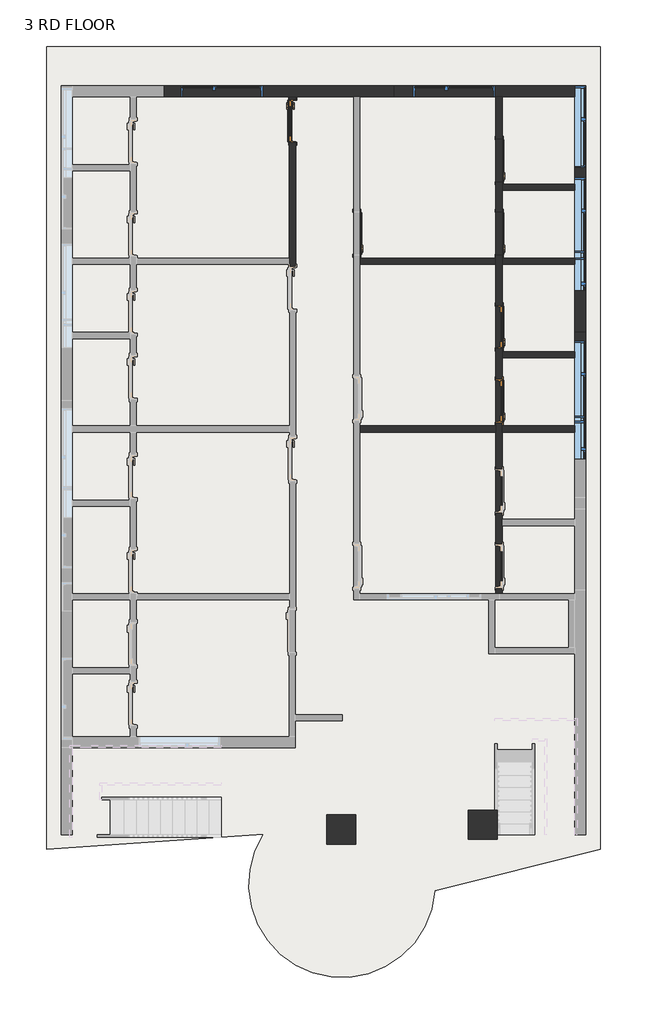
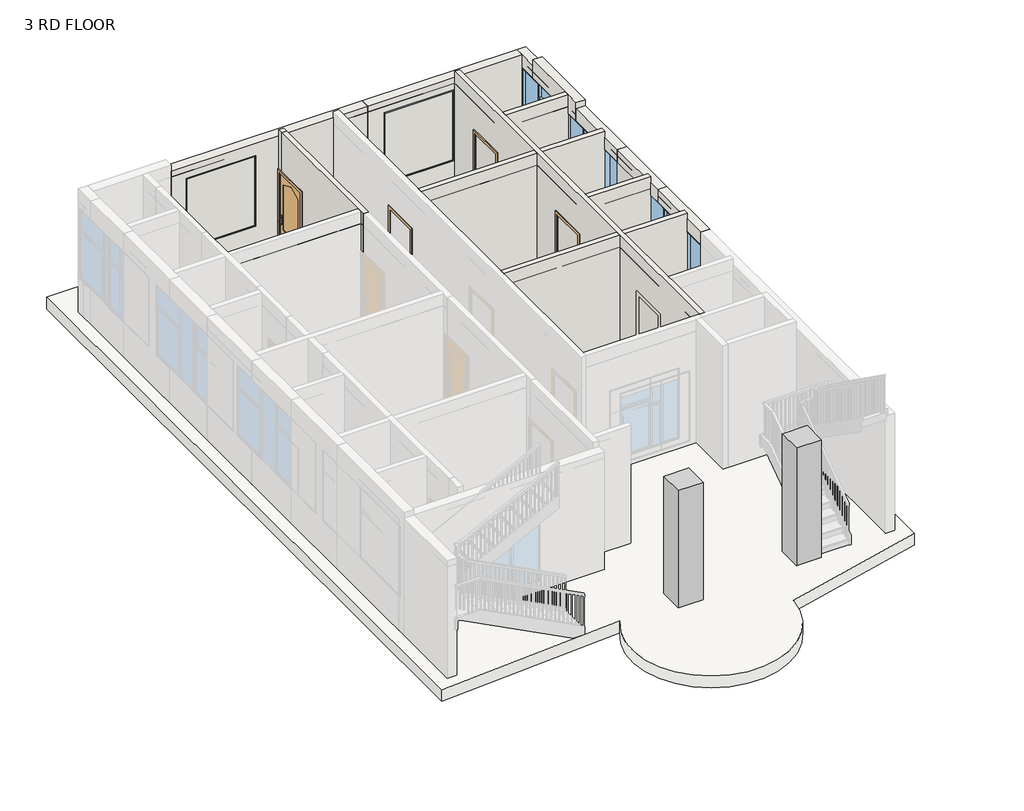
# One storey, part 3 of 5: 33 walls, 7 windows, 6 doors, 2 columns, 1 slab.
"""IFC4 building model written with IfcOpenShell, lengths in millimetres."""

from ifc_helpers import new_model, si_unit, point, frame, frame_2d, origin, place, context, project, spatial, polyline, circle_curve, trimmed, segment, composite_curve, outline, extrude, faceted_brep, transform, mapped, element, save
from components import column_08700e81, door_346b4a94, m_window_casement_double_sidelight_1702_x_1829mm_c8b42c7f

model = new_model("IFC4")

# Units and contexts
model_context = context("Model", 3, world=origin())
ifc_project = project(units=[si_unit("LENGTHUNIT", "METRE", prefix="MILLI")], contexts=[model_context])

# Site, building, storey
site = spatial("IfcSite", under=ifc_project)
building = spatial("IfcBuilding", under=site)
storey = spatial("IfcBuildingStorey", under=building, Name="3 RD FLOOR", Elevation=9601.2)

# Columns
placement = place(None, origin())
element("IfcColumn", 1, ObjectType="Rectangular Column : 24\" x 24\"", at=placement, inside=storey, context=model_context, shape_type="SweptSolid", body=[
    extrude(outline(polyline([(2657.4891134, -7132.8082131), (2657.4891134, -7742.4082131), (2047.8891134, -7742.4082131), (2047.8891134, -7132.8082131), (2657.4891134, -7132.8082131)])), frame((0.0, 0.0, 9601.2), z_axis=(0.0, 0.0, 1.0), x_axis=(1.0, 0.0, 0.0)), (0.0, 0.0, 1.0), 3048.0),
])
column_shape = column_08700e81(model_context)
element("IfcColumn", 2, ObjectType="Rectangular Column : 24\" x 24\"", at=placement, inside=storey, context=model_context, shape_type="MappedRepresentation", body=[
    mapped(column_shape, transform((-606.4108866, -7539.2082131, 0.0), x_axis=(1.0, 0.0, 0.0), y_axis=(0.0, 1.0, 0.0), z_axis=(0.0, 0.0, 1.0))),
])

# Doors
door_shape = door_346b4a94(model_context)
element("IfcDoor", 3, ObjectType="2'10\"X7'", at=placement, inside=storey, context=model_context, shape_type="MappedRepresentation", body=[
    mapped(door_shape, transform((2698.7641134, 6449.4399728, 9601.2), x_axis=(0.0, -1.0, 0.0), y_axis=(1.0, 0.0, 0.0), z_axis=(0.0, 0.0, 1.0))),
])
element("IfcDoor", 4, ObjectType="2'10\"X7'", at=placement, inside=storey, context=model_context, shape_type="MappedRepresentation", body=[
    mapped(door_shape, transform((2698.7641134, 4925.4399728, 9601.2), x_axis=(0.0, -1.0, 0.0), y_axis=(1.0, 0.0, 0.0), z_axis=(0.0, 0.0, 1.0))),
])
element("IfcDoor", 5, ObjectType="2'10\"X7'", at=placement, inside=storey, context=model_context, shape_type="MappedRepresentation", body=[
    mapped(door_shape, transform((2698.7641134, 2969.6399728, 9601.2), x_axis=(0.0, -1.0, 0.0), y_axis=(1.0, 0.0, 0.0), z_axis=(0.0, 0.0, 1.0))),
])
element("IfcDoor", 6, ObjectType="2'10\"X7'", at=placement, inside=storey, context=model_context, shape_type="MappedRepresentation", body=[
    mapped(door_shape, transform((2698.7641134, 1420.2399728, 9601.2), x_axis=(0.0, -1.0, 0.0), y_axis=(1.0, 0.0, 0.0), z_axis=(0.0, 0.0, 1.0))),
])
element("IfcDoor", 7, ObjectType="2'10\"X7'", at=placement, inside=storey, context=model_context, shape_type="MappedRepresentation", body=[
    mapped(door_shape, transform((-273.0358866, 4925.4399728, 9601.2), x_axis=(0.0, -1.0, 0.0), y_axis=(1.0, 0.0, 0.0), z_axis=(0.0, 0.0, 1.0))),
])
element("IfcDoor", 8, ObjectType="2'10\"X7'", at=placement, inside=storey, context=model_context, shape_type="MappedRepresentation", body=[
    mapped(door_shape, transform((-1625.5858866, 7274.3310623, 9601.2), x_axis=(0.0, 1.0, 0.0), y_axis=(-1.0, 0.0, 0.0), z_axis=(0.0, 0.0, 1.0))),
])

# Slab
element("IfcSlab", 9, ObjectType="Generic - 12\"", at=placement, inside=storey, context=model_context, shape_type="SweptSolid", body=[
    extrude(outline(composite_curve([segment(polyline([(4815.1311655, 8833.6177996), (4815.1311655, -7955.7822004), (1352.4742985, -8819.1195216)]), True, "CONTINUOUS"), segment(trimmed(circle_curve(frame_2d((-589.5644815, -8685.9789369)), 1946.5972974), [point((1352.4742985, -8819.1195216))], [point((-2230.3861756, -7638.6274169))], False, "CARTESIAN"), True, "CONTINUOUS"), segment(polyline([(-2230.3861756, -7638.6274169), (-6765.9108866, -7955.7822004), (-6765.9108866, 8833.6177996), (4815.1311655, 8833.6177996)]), True, "CONTINUOUS")], self_intersect=False)), frame((0.0, 0.0, 9296.4), z_axis=(0.0, 0.0, 1.0), x_axis=(1.0, 0.0, 0.0)), (0.0, 0.0, 1.0), 304.8),
])

# Walls
element("IfcWall", 10, ObjectType="Generic - 4.5\"", at=placement, inside=storey, context=model_context, shape_type="Brep", body=[
    faceted_brep([(-1685.9108866, 7655.3310623, 12801.6), (-1685.9108866, 7782.9399728, 12801.6), (-1685.9108866, 7782.9399728, 9601.2), (-1685.9108866, 7731.1310623, 9601.2), (-1685.9108866, 7731.1310623, 11759.8), (-1685.9108866, 7655.3310623, 11759.8), (-1685.9108866, 7655.3310623, 12496.8), (-1558.9108866, 7782.9399728, 12801.6), (-1558.9108866, 7655.3310623, 12801.6), (-1558.9108866, 7655.3310623, 12496.8), (-1558.9108866, 7655.3310623, 11759.8), (-1558.9108866, 7731.1310623, 11759.8), (-1558.9108866, 7731.1310623, 9601.2), (-1558.9108866, 7782.9399728, 9601.2)], [[[0, 1, 2, 3, 4, 5, 6]], [[7, 8, 9, 10, 11, 12, 13]], [[2, 13, 12, 3]], [[1, 0, 8, 7]], [[11, 4, 3, 12]], [[4, 11, 10, 5]], [[8, 0, 6, 5, 10, 9]], [[1, 7, 13, 2]]]),
])
element("IfcWall", 11, ObjectType="Generic - 4.5\"", at=placement, inside=storey, context=model_context, shape_type="Brep", body=[
    faceted_brep([(-1685.9108866, 4182.2008884, 12801.6), (-1685.9108866, 4277.7399728, 12801.6), (-1685.9108866, 4404.7399728, 12801.6), (-1685.9108866, 7655.3310623, 12801.6), (-1685.9108866, 7655.3310623, 12496.8), (-1685.9108866, 7655.3310623, 11759.8), (-1685.9108866, 6817.5310623, 11759.8), (-1685.9108866, 6817.5310623, 9601.2), (-1685.9108866, 4404.7399728, 9601.2), (-1685.9108866, 4277.7399728, 9601.2), (-1685.9108866, 4232.6008884, 9601.2), (-1685.9108866, 4232.6008884, 11759.8), (-1685.9108866, 4182.2008884, 11759.8), (-1558.9108866, 7655.3310623, 12801.6), (-1558.9108866, 4182.2008884, 12801.6), (-1558.9108866, 4182.2008884, 11759.8), (-1558.9108866, 4232.6008884, 11759.8), (-1558.9108866, 4232.6008884, 9601.2), (-1558.9108866, 6817.5310623, 9601.2), (-1558.9108866, 6817.5310623, 11759.8), (-1558.9108866, 7655.3310623, 11759.8), (-1558.9108866, 7655.3310623, 12496.8), (-1685.4871817, 4182.2008884, 12801.6), (-1685.4871817, 4182.2008884, 11759.8)], [[[0, 1, 2, 3, 4, 5, 6, 7, 8, 9, 10, 11, 12]], [[13, 14, 15, 16, 17, 18, 19, 20, 21]], [[17, 10, 9, 8, 7, 18]], [[3, 2, 1, 0, 22, 14, 13]], [[16, 11, 10, 17]], [[11, 16, 15, 23, 12]], [[19, 6, 5, 20]], [[6, 19, 18, 7]], [[14, 22, 0, 12, 23, 15]], [[3, 13, 21, 20, 5, 4]]]),
])
element("IfcWall", 12, ObjectType="Generic - 4.5\"", at=placement, inside=storey, context=model_context, shape_type="Brep", body=[
    faceted_brep([(2632.0891134, -2605.6600272, 12801.6), (2632.0891134, 772.5399728, 12801.6), (2632.0891134, 899.5399728, 12801.6), (2632.0891134, 4277.7399728, 12801.6), (2632.0891134, 4404.7399728, 12801.6), (2632.0891134, 7782.9399728, 12801.6), (2632.0891134, 7782.9399728, 9601.2), (2632.0891134, 6906.2399728, 9601.2), (2632.0891134, 6906.2399728, 11759.8), (2632.0891134, 5992.6399728, 11759.8), (2632.0891134, 5992.6399728, 9601.2), (2632.0891134, 5382.2399728, 9601.2), (2632.0891134, 5382.2399728, 11759.8), (2632.0891134, 4468.6399728, 11759.8), (2632.0891134, 4468.6399728, 9601.2), (2632.0891134, 4404.7399728, 9601.2), (2632.0891134, 4277.7399728, 9601.2), (2632.0891134, 3426.4399728, 9601.2), (2632.0891134, 3426.4399728, 11759.8), (2632.0891134, 2512.8399728, 11759.8), (2632.0891134, 2512.8399728, 9601.2), (2632.0891134, 1877.0399728, 9601.2), (2632.0891134, 1877.0399728, 11759.8), (2632.0891134, 963.4399728, 11759.8), (2632.0891134, 963.4399728, 9601.2), (2632.0891134, 899.5399728, 9601.2), (2632.0891134, 772.5399728, 9601.2), (2632.0891134, -2.5600272, 9601.2), (2632.0891134, -2.5600272, 11759.8), (2632.0891134, -916.1600272, 11759.8), (2632.0891134, -916.1600272, 9601.2), (2632.0891134, -1577.3600272, 9601.2), (2632.0891134, -1577.3600272, 11759.8), (2632.0891134, -2490.9600272, 11759.8), (2632.0891134, -2490.9600272, 9601.2), (2632.0891134, -2605.6600272, 9601.2), (2632.0891134, -2605.6600272, 12496.8), (2759.0891134, 7782.9399728, 12801.6), (2759.0891134, 5954.1399728, 12801.6), (2759.0891134, 5827.1399728, 12801.6), (2759.0891134, 4404.7399728, 12801.6), (2759.0891134, 4277.7399728, 12801.6), (2759.0891134, 2448.9399728, 12801.6), (2759.0891134, 2321.9399728, 12801.6), (2759.0891134, 899.5399728, 12801.6), (2759.0891134, 772.5399728, 12801.6), (2759.0891134, -1056.2600272, 12801.6), (2759.0891134, -1183.2600272, 12801.6), (2759.0891134, -2605.6600272, 12801.6), (2759.0891134, -2605.6600272, 9601.2), (2759.0891134, -2490.9600272, 9601.2), (2759.0891134, -2490.9600272, 11759.8), (2759.0891134, -1577.3600272, 11759.8), (2759.0891134, -1577.3600272, 9601.2), (2759.0891134, -1183.2600272, 9601.2), (2759.0891134, -1056.2600272, 9601.2), (2759.0891134, -916.1600272, 9601.2), (2759.0891134, -916.1600272, 11759.8), (2759.0891134, -2.5600272, 11759.8), (2759.0891134, -2.5600272, 9601.2), (2759.0891134, 772.5399728, 9601.2), (2759.0891134, 899.5399728, 9601.2), (2759.0891134, 963.4399728, 9601.2), (2759.0891134, 963.4399728, 11759.8), (2759.0891134, 1877.0399728, 11759.8), (2759.0891134, 1877.0399728, 9601.2), (2759.0891134, 2321.9399728, 9601.2), (2759.0891134, 2448.9399728, 9601.2), (2759.0891134, 2512.8399728, 9601.2), (2759.0891134, 2512.8399728, 11759.8), (2759.0891134, 3426.4399728, 11759.8), (2759.0891134, 3426.4399728, 9601.2), (2759.0891134, 4277.7399728, 9601.2), (2759.0891134, 4404.7399728, 9601.2), (2759.0891134, 4468.6399728, 9601.2), (2759.0891134, 4468.6399728, 11759.8), (2759.0891134, 5382.2399728, 11759.8), (2759.0891134, 5382.2399728, 9601.2), (2759.0891134, 5827.1399728, 9601.2), (2759.0891134, 5954.1399728, 9601.2), (2759.0891134, 5992.6399728, 9601.2), (2759.0891134, 5992.6399728, 11759.8), (2759.0891134, 6906.2399728, 11759.8), (2759.0891134, 6906.2399728, 9601.2), (2759.0891134, 7782.9399728, 9601.2), (2695.5891134, -2605.6600272, 9601.2)], [[[0, 1, 2, 3, 4, 5, 6, 7, 8, 9, 10, 11, 12, 13, 14, 15, 16, 17, 18, 19, 20, 21, 22, 23, 24, 25, 26, 27, 28, 29, 30, 31, 32, 33, 34, 35, 36]], [[37, 38, 39, 40, 41, 42, 43, 44, 45, 46, 47, 48, 49, 50, 51, 52, 53, 54, 55, 56, 57, 58, 59, 60, 61, 62, 63, 64, 65, 66, 67, 68, 69, 70, 71, 72, 73, 74, 75, 76, 77, 78, 79, 80, 81, 82, 83, 84]], [[6, 84, 83, 7]], [[10, 80, 79, 78, 77, 11]], [[14, 74, 73, 72, 71, 17, 16, 15]], [[20, 68, 67, 66, 65, 21]], [[24, 62, 61, 60, 59, 27, 26, 25]], [[30, 56, 55, 54, 53, 31]], [[49, 85, 35, 34, 50]], [[5, 4, 3, 2, 1, 0, 48, 47, 46, 45, 44, 43, 42, 41, 40, 39, 38, 37]], [[6, 5, 37, 84]], [[9, 81, 80, 10]], [[81, 9, 8, 82]], [[82, 8, 7, 83]], [[14, 13, 75, 74]], [[13, 12, 76, 75]], [[12, 11, 77, 76]], [[19, 69, 68, 20]], [[69, 19, 18, 70]], [[70, 18, 17, 71]], [[23, 63, 62, 24]], [[63, 23, 22, 64]], [[64, 22, 21, 65]], [[29, 57, 56, 30]], [[57, 29, 28, 58]], [[58, 28, 27, 59]], [[33, 51, 50, 34]], [[51, 33, 32, 52]], [[52, 32, 31, 53]], [[35, 85, 49, 48, 0, 36]]]),
])
element("IfcWall", 13, ObjectType="Generic - 4.5\"", at=placement, inside=storey, context=model_context, shape_type="SweptSolid", body=[
    extrude(outline(polyline([(2632.0891134, 4277.7399728), (-212.7108866, 4277.7399728), (-212.7108866, 4404.7399728), (2632.0891134, 4404.7399728), (2632.0891134, 4277.7399728)])), frame((0.0, 0.0, 9601.2), z_axis=(0.0, 0.0, 1.0), x_axis=(1.0, 0.0, 0.0)), (0.0, 0.0, 1.0), 3200.4),
])
element("IfcWall", 14, ObjectType="Generic - 4.5\"", at=placement, inside=storey, context=model_context, shape_type="SweptSolid", body=[
    extrude(outline(polyline([(2632.0891134, 772.5399728), (-212.7108866, 772.5399728), (-212.7108866, 899.5399728), (2632.0891134, 899.5399728), (2632.0891134, 772.5399728)])), frame((0.0, 0.0, 9601.2), z_axis=(0.0, 0.0, 1.0), x_axis=(1.0, 0.0, 0.0)), (0.0, 0.0, 1.0), 3200.4),
])
element("IfcWall", 15, ObjectType="Generic - 4.5\"", at=placement, inside=storey, context=model_context, shape_type="SweptSolid", body=[
    extrude(outline(polyline([(4281.587404, 5827.1399728), (2759.0891134, 5827.1399728), (2759.0891134, 5954.1399728), (4281.587404, 5954.1399728), (4281.587404, 5827.1399728)])), frame((0.0, 0.0, 9601.2), z_axis=(0.0, 0.0, 1.0), x_axis=(1.0, 0.0, 0.0)), (0.0, 0.0, 1.0), 3200.4),
])
element("IfcWall", 16, ObjectType="Generic - 4.5\"", at=placement, inside=storey, context=model_context, shape_type="SweptSolid", body=[
    extrude(outline(polyline([(4283.9989713, 4277.7399728), (2759.0891134, 4277.7399728), (2759.0891134, 4404.7399728), (4283.9989713, 4404.7399728), (4283.9989713, 4277.7399728)])), frame((0.0, 0.0, 9601.2), z_axis=(0.0, 0.0, 1.0), x_axis=(1.0, 0.0, 0.0)), (0.0, 0.0, 1.0), 3200.4),
])
element("IfcWall", 17, ObjectType="Generic - 4.5\"", at=placement, inside=storey, context=model_context, shape_type="SweptSolid", body=[
    extrude(outline(polyline([(4281.0767915, 2321.9399728), (2759.0891134, 2321.9399728), (2759.0891134, 2448.9399728), (4281.0767915, 2448.9399728), (4281.0767915, 2321.9399728)])), frame((0.0, 0.0, 9601.2), z_axis=(0.0, 0.0, 1.0), x_axis=(1.0, 0.0, 0.0)), (0.0, 0.0, 1.0), 3200.4),
])
element("IfcWall", 18, ObjectType="Generic - 4.5\"", at=placement, inside=storey, context=model_context, shape_type="SweptSolid", body=[
    extrude(outline(polyline([(4283.0918814, 772.5399728), (2759.0891134, 772.5399728), (2759.0891134, 899.5399728), (4283.0918814, 899.5399728), (4283.0918814, 772.5399728)])), frame((0.0, 0.0, 9601.2), z_axis=(0.0, 0.0, 1.0), x_axis=(1.0, 0.0, 0.0)), (0.0, 0.0, 1.0), 3200.4),
])
element("IfcWall", 19, ObjectType="Generic - 4.5\"", at=placement, inside=storey, context=model_context, shape_type="SweptSolid", body=[
    extrude(outline(polyline([(-1685.9108866, 4277.7399728), (-4886.3108866, 4277.7399728), (-4886.3108866, 4404.7399728), (-1685.9108866, 4404.7399728), (-1685.9108866, 4277.7399728)])), frame((0.0, 0.0, 9601.2), z_axis=(0.0, 0.0, 1.0), x_axis=(1.0, 0.0, 0.0)), (0.0, 0.0, 1.0), 2895.6),
])
element("IfcWall", 20, ObjectType="Generic - 4.5\"", at=placement, inside=storey, context=model_context, shape_type="SweptSolid", body=[
    extrude(outline(polyline([(7782.9399728, 12496.8), (7782.9399728, 9601.2), (7731.1310623, 9601.2), (7731.1310623, 11759.8), (7655.3310623, 11759.8), (7655.3310623, 12496.8), (7782.9399728, 12496.8)])), frame((-1685.9108866, 0.0, 0.0), z_axis=(1.0, 0.0, 0.0), x_axis=(0.0, 1.0, 0.0)), (0.0, 0.0, 1.0), 127.0),
])
element("IfcWall", 21, ObjectType="Generic - 4.5\"", at=placement, inside=storey, context=model_context, shape_type="Brep", body=[
    faceted_brep([(-1685.9108866, 4182.2008884, 12496.8), (-1685.9108866, 4277.7399728, 12496.8), (-1685.9108866, 4404.7399728, 12496.8), (-1685.9108866, 7655.3310623, 12496.8), (-1685.9108866, 7655.3310623, 11759.8), (-1685.9108866, 6817.5310623, 11759.8), (-1685.9108866, 6817.5310623, 9601.2), (-1685.9108866, 4404.7399728, 9601.2), (-1685.9108866, 4277.7399728, 9601.2), (-1685.9108866, 4232.6008884, 9601.2), (-1685.9108866, 4232.6008884, 11759.8), (-1685.9108866, 4182.2008884, 11759.8), (-1558.9108866, 7655.3310623, 12496.8), (-1558.9108866, 4182.2008884, 12496.8), (-1558.9108866, 4182.2008884, 11759.8), (-1558.9108866, 4232.6008884, 11759.8), (-1558.9108866, 4232.6008884, 9601.2), (-1558.9108866, 6817.5310623, 9601.2), (-1558.9108866, 6817.5310623, 11759.8), (-1558.9108866, 7655.3310623, 11759.8), (-1685.4871817, 4182.2008884, 12496.8), (-1685.4871817, 4182.2008884, 11759.8)], [[[0, 1, 2, 3, 4, 5, 6, 7, 8, 9, 10, 11]], [[12, 13, 14, 15, 16, 17, 18, 19]], [[16, 9, 8, 7, 6, 17]], [[13, 20, 0, 11, 21, 14]], [[3, 12, 19, 4]], [[3, 2, 1, 0, 20, 13, 12]], [[18, 5, 4, 19]], [[5, 18, 17, 6]], [[15, 10, 9, 16]], [[10, 15, 14, 21, 11]]]),
])
element("IfcWall", 22, ObjectType="Generic - 4.5\"", at=placement, inside=storey, context=model_context, shape_type="Brep", body=[
    faceted_brep([(2632.0891134, 7782.9399728, 9601.2), (2632.0891134, 4404.7399728, 9601.2), (2632.0891134, 4277.7399728, 9601.2), (2632.0891134, 899.5399728, 9601.2), (2632.0891134, 772.5399728, 9601.2), (2632.0891134, -2605.6600272, 9601.2), (2632.0891134, -2605.6600272, 12496.8), (2632.0891134, 772.5399728, 12496.8), (2632.0891134, 899.5399728, 12496.8), (2632.0891134, 4277.7399728, 12496.8), (2632.0891134, 4404.7399728, 12496.8), (2632.0891134, 7782.9399728, 12496.8), (2759.0891134, 7782.9399728, 9601.2), (2759.0891134, 7782.9399728, 12496.8), (2759.0891134, 5954.1399728, 12496.8), (2759.0891134, 5827.1399728, 12496.8), (2759.0891134, 4404.7399728, 12496.8), (2759.0891134, 4277.7399728, 12496.8), (2759.0891134, 2448.9399728, 12496.8), (2759.0891134, 2321.9399728, 12496.8), (2759.0891134, 899.5399728, 12496.8), (2759.0891134, 772.5399728, 12496.8), (2759.0891134, -1056.2600272, 12496.8), (2759.0891134, -1183.2600272, 12496.8), (2759.0891134, -2605.6600272, 12496.8), (2759.0891134, -2605.6600272, 9601.2), (2759.0891134, -1183.2600272, 9601.2), (2759.0891134, -1056.2600272, 9601.2), (2759.0891134, 772.5399728, 9601.2), (2759.0891134, 899.5399728, 9601.2), (2759.0891134, 2321.9399728, 9601.2), (2759.0891134, 2448.9399728, 9601.2), (2759.0891134, 4277.7399728, 9601.2), (2759.0891134, 4404.7399728, 9601.2), (2759.0891134, 5827.1399728, 9601.2), (2759.0891134, 5954.1399728, 9601.2), (2695.5891134, -2605.6600272, 9601.2), (2695.5891134, -2605.6600272, 12496.8)], [[[0, 1, 2, 3, 4, 5, 6, 7, 8, 9, 10, 11]], [[12, 13, 14, 15, 16, 17, 18, 19, 20, 21, 22, 23, 24, 25, 26, 27, 28, 29, 30, 31, 32, 33, 34, 35]], [[5, 4, 3, 2, 1, 0, 12, 35, 34, 33, 32, 31, 30, 29, 28, 27, 26, 25, 36]], [[0, 11, 13, 12]], [[6, 5, 36, 25, 24, 37]], [[11, 10, 9, 8, 7, 6, 37, 24, 23, 22, 21, 20, 19, 18, 17, 16, 15, 14, 13]]]),
])
element("IfcWall", 23, ObjectType="Generic - 4.5\"", at=placement, inside=storey, context=model_context, shape_type="SweptSolid", body=[
    extrude(outline(polyline([(2632.0891134, 4277.7399728), (-212.7108866, 4277.7399728), (-212.7108866, 4404.7399728), (2632.0891134, 4404.7399728), (2632.0891134, 4277.7399728)])), frame((0.0, 0.0, 9601.2), z_axis=(0.0, 0.0, 1.0), x_axis=(1.0, 0.0, 0.0)), (0.0, 0.0, 1.0), 2895.6),
])
element("IfcWall", 24, ObjectType="Generic - 4.5\"", at=placement, inside=storey, context=model_context, shape_type="SweptSolid", body=[
    extrude(outline(polyline([(2632.0891134, 772.5399728), (-212.7108866, 772.5399728), (-212.7108866, 899.5399728), (2632.0891134, 899.5399728), (2632.0891134, 772.5399728)])), frame((0.0, 0.0, 9601.2), z_axis=(0.0, 0.0, 1.0), x_axis=(1.0, 0.0, 0.0)), (0.0, 0.0, 1.0), 2895.6),
])
element("IfcWall", 25, ObjectType="Generic - 4.5\"", at=placement, inside=storey, context=model_context, shape_type="SweptSolid", body=[
    extrude(outline(polyline([(4281.587404, 5827.1399728), (2759.0891134, 5827.1399728), (2759.0891134, 5954.1399728), (4281.587404, 5954.1399728), (4281.587404, 5827.1399728)])), frame((0.0, 0.0, 9601.2), z_axis=(0.0, 0.0, 1.0), x_axis=(1.0, 0.0, 0.0)), (0.0, 0.0, 1.0), 2895.6),
])
element("IfcWall", 26, ObjectType="Generic - 4.5\"", at=placement, inside=storey, context=model_context, shape_type="SweptSolid", body=[
    extrude(outline(polyline([(4283.9989713, 4277.7399728), (2759.0891134, 4277.7399728), (2759.0891134, 4404.7399728), (4283.9989713, 4404.7399728), (4283.9989713, 4277.7399728)])), frame((0.0, 0.0, 9601.2), z_axis=(0.0, 0.0, 1.0), x_axis=(1.0, 0.0, 0.0)), (0.0, 0.0, 1.0), 2895.6),
])
element("IfcWall", 27, ObjectType="Generic - 4.5\"", at=placement, inside=storey, context=model_context, shape_type="SweptSolid", body=[
    extrude(outline(polyline([(4281.0767915, 2321.9399728), (2759.0891134, 2321.9399728), (2759.0891134, 2448.9399728), (4281.0767915, 2448.9399728), (4281.0767915, 2321.9399728)])), frame((0.0, 0.0, 9601.2), z_axis=(0.0, 0.0, 1.0), x_axis=(1.0, 0.0, 0.0)), (0.0, 0.0, 1.0), 2895.6),
])
element("IfcWall", 28, ObjectType="Generic - 4.5\"", at=placement, inside=storey, context=model_context, shape_type="SweptSolid", body=[
    extrude(outline(polyline([(4283.0918814, 772.5399728), (2759.0891134, 772.5399728), (2759.0891134, 899.5399728), (4283.0918814, 899.5399728), (4283.0918814, 772.5399728)])), frame((0.0, 0.0, 9601.2), z_axis=(0.0, 0.0, 1.0), x_axis=(1.0, 0.0, 0.0)), (0.0, 0.0, 1.0), 2895.6),
])
element("IfcWall", 29, ObjectType="Generic - 9\"", at=placement, inside=storey, context=model_context, shape_type="Brep", body=[
    faceted_brep([(-4318.2603585, 7782.9399728, 12649.2), (-4318.2603585, 7782.9399728, 12496.8), (-4318.2603585, 7782.9399728, 9601.2), (-1685.9108866, 7782.9399728, 9601.2), (-1558.9108866, 7782.9399728, 9601.2), (-339.7108866, 7782.9399728, 9601.2), (-212.7108866, 7782.9399728, 9601.2), (496.3553976, 7782.9399728, 9601.2), (496.3553976, 7782.9399728, 12496.8), (496.3553976, 7782.9399728, 12649.2), (-2248.1603585, 7782.9399728, 12330.0), (-2248.1603585, 7782.9399728, 10501.2), (-3949.9603585, 7782.9399728, 10501.2), (-3949.9603585, 7782.9399728, 12330.0), (-4318.2603585, 8011.5399728, 9601.2), (-4318.2603585, 8011.5399728, 12496.8), (-4318.2603585, 8011.5399728, 12649.2), (496.3553976, 8011.5399728, 12649.2), (496.3553976, 8011.5399728, 12496.8), (496.3553976, 8011.5399728, 9601.2), (-2248.1603585, 8011.5399728, 12330.0), (-3949.9603585, 8011.5399728, 12330.0), (-3949.9603585, 8011.5399728, 10501.2), (-2248.1603585, 8011.5399728, 10501.2)], [[[0, 1, 2, 3, 4, 5, 6, 7, 8, 9], [10, 11, 12, 13]], [[14, 15, 16, 17, 18, 19], [20, 21, 22, 23]], [[7, 6, 5, 4, 3, 2, 14, 19]], [[0, 9, 17, 16]], [[11, 10, 20, 23]], [[12, 11, 23, 22]], [[13, 12, 22, 21]], [[10, 13, 21, 20]], [[7, 19, 18, 17, 9, 8]], [[0, 16, 15, 14, 2, 1]]]),
])
element("IfcWall", 30, ObjectType="Generic - 9\"", at=placement, inside=storey, context=model_context, shape_type="Brep", body=[
    faceted_brep([(496.3553976, 7782.9399728, 9601.2), (2632.0891134, 7782.9399728, 9601.2), (2759.0891134, 7782.9399728, 9601.2), (4283.0891134, 7782.9399728, 9601.2), (4283.0891134, 7782.9399728, 10501.2), (4281.587404, 7782.9399728, 10501.2), (4281.587404, 7782.9399728, 12330.0), (4283.0891134, 7782.9399728, 12330.0), (4283.0891134, 7782.9399728, 12649.2), (496.3553976, 7782.9399728, 12649.2), (496.3553976, 7782.9399728, 12496.8), (2606.6891134, 7782.9399728, 12330.0), (2606.6891134, 7782.9399728, 10501.2), (904.8891134, 7782.9399728, 10501.2), (904.8891134, 7782.9399728, 12330.0), (4283.0891134, 8011.5399728, 9601.2), (496.3553976, 8011.5399728, 9601.2), (496.3553976, 8011.5399728, 12496.8), (496.3553976, 8011.5399728, 12649.2), (4283.0891134, 8011.5399728, 12649.2), (4283.0891134, 8011.5399728, 12496.8), (2606.6891134, 8011.5399728, 10501.2), (2606.6891134, 8011.5399728, 12330.0), (904.8891134, 8011.5399728, 12330.0), (904.8891134, 8011.5399728, 10501.2), (4283.0891134, 7998.8399728, 12330.0), (4283.0891134, 7998.8399728, 10501.2), (4281.587404, 7998.8399728, 10501.2), (4281.587404, 7998.8399728, 12330.0)], [[[0, 1, 2, 3, 4, 5, 6, 7, 8, 9, 10], [11, 12, 13, 14]], [[15, 16, 17, 18, 19, 20], [21, 22, 23, 24]], [[3, 2, 1, 0, 16, 15]], [[9, 8, 19, 18]], [[12, 11, 22, 21]], [[13, 12, 21, 24]], [[14, 13, 24, 23]], [[11, 14, 23, 22]], [[9, 18, 17, 16, 0, 10]], [[3, 15, 20, 19, 8, 7, 25, 26, 4]], [[27, 28, 6, 5]], [[27, 5, 4, 26]], [[28, 27, 26, 25]], [[6, 28, 25, 7]]]),
])
element("IfcWall", 31, ObjectType="Generic - 9\"", at=placement, inside=storey, context=model_context, shape_type="Brep", body=[
    faceted_brep([(4283.0891134, 7782.9399728, 9601.2), (4283.0891134, 7325.7399728, 9601.2), (4283.0891134, 7325.7399728, 10501.2), (4283.0891134, 7782.9399728, 10501.2), (4511.6891134, 7325.7399728, 9601.2), (4511.6891134, 7782.9399728, 9601.2), (4511.6891134, 7782.9399728, 10501.2), (4511.6891134, 7325.7399728, 10501.2), (4510.187404, 7325.7399728, 9601.2), (4510.187404, 7325.7399728, 10501.2)], [[[0, 1, 2, 3]], [[4, 5, 6, 7]], [[1, 0, 5, 4, 8]], [[3, 2, 9, 7, 6]], [[1, 8, 4, 7, 9, 2]], [[5, 0, 3, 6]]]),
    faceted_brep([(4283.0891134, 7325.7399728, 12649.2), (4283.0891134, 7782.9399728, 12649.2), (4283.0891134, 8011.5399728, 12649.2), (4283.0891134, 8011.5399728, 12496.8), (4283.0891134, 7782.9399728, 12496.8), (4283.0891134, 7782.9399728, 12330.0), (4283.0891134, 7325.7399728, 12330.0), (4511.6891134, 8011.5399728, 12649.2), (4511.6891134, 7325.7399728, 12649.2), (4511.6891134, 7325.7399728, 12330.0), (4511.6891134, 7782.9399728, 12330.0), (4511.6891134, 7782.9399728, 12496.8), (4511.6891134, 8011.5399728, 12496.8), (4510.187404, 7325.7399728, 12330.0)], [[[0, 1, 2, 3, 4, 5, 6]], [[7, 8, 9, 10, 11, 12]], [[2, 1, 0, 8, 7]], [[6, 5, 10, 9, 13]], [[8, 0, 6, 13, 9]], [[12, 11, 4, 3]], [[4, 11, 10, 5]], [[3, 2, 7, 12]]]),
])
element("IfcWall", 32, ObjectType="Generic - 9\"", at=placement, inside=storey, context=model_context, shape_type="Brep", body=[
    faceted_brep([(4281.587404, 7325.7399728, 9601.2), (4281.587404, 5954.1399728, 9601.2), (4281.587404, 5827.1399728, 9601.2), (4281.587404, 5490.9915892, 9601.2), (4281.587404, 5490.9915892, 10501.2), (4281.587404, 6087.8915892, 10501.2), (4281.587404, 6087.8915892, 12330.0), (4281.587404, 5490.9915892, 12330.0), (4281.587404, 5490.9915892, 12801.6), (4281.587404, 5827.1399728, 12801.6), (4281.587404, 5954.1399728, 12801.6), (4281.587404, 7325.7399728, 12801.6), (4281.587404, 7325.7399728, 12330.0), (4281.587404, 6297.0399728, 12330.0), (4281.587404, 6297.0399728, 10501.2), (4281.587404, 7325.7399728, 10501.2), (4510.187404, 5490.9915892, 9601.2), (4510.187404, 7325.7399728, 9601.2), (4510.187404, 7325.7399728, 10501.2), (4510.187404, 6297.0399728, 10501.2), (4510.187404, 6297.0399728, 12330.0), (4510.187404, 7325.7399728, 12330.0), (4510.187404, 7325.7399728, 12801.6), (4510.187404, 5490.9915892, 12801.6), (4510.187404, 5490.9915892, 12330.0), (4510.187404, 6087.8915892, 12330.0), (4510.187404, 6087.8915892, 10501.2), (4510.187404, 5490.9915892, 10501.2), (4283.0891134, 7325.7399728, 9601.2), (4283.9989713, 5490.9915892, 9601.2), (4283.0891134, 7325.7399728, 10501.2), (4283.0891134, 7325.7399728, 12330.0), (4283.9989713, 5490.9915892, 10501.2), (4283.9989713, 5490.9915892, 12330.0)], [[[0, 1, 2, 3, 4, 5, 6, 7, 8, 9, 10, 11, 12, 13, 14, 15]], [[16, 17, 18, 19, 20, 21, 22, 23, 24, 25, 26, 27]], [[3, 2, 1, 0, 28, 17, 16, 29]], [[11, 10, 9, 8, 23, 22]], [[13, 20, 19, 14]], [[14, 19, 18, 30, 15]], [[20, 13, 12, 31, 21]], [[26, 5, 4, 32, 27]], [[5, 26, 25, 6]], [[6, 25, 24, 33, 7]], [[23, 8, 7, 33, 24]], [[3, 29, 16, 27, 32, 4]], [[11, 22, 21, 31, 12]], [[17, 28, 0, 15, 30, 18]]]),
])
element("IfcWall", 33, ObjectType="Generic - 9\"", at=placement, inside=storey, context=model_context, shape_type="Brep", body=[
    faceted_brep([(4283.9989713, 3730.8359967, 12649.2), (4283.9989713, 5490.9915892, 12649.2), (4283.9989713, 5490.9915892, 12330.0), (4283.9989713, 3730.8359967, 12330.0), (4512.5989713, 5490.9915892, 12649.2), (4512.5989713, 3730.8359967, 12649.2), (4512.5989713, 3730.8359967, 12330.0), (4512.5989713, 5490.9915892, 12330.0), (4509.6767915, 3730.8359967, 12649.2), (4510.187404, 5490.9915892, 12330.0), (4509.6767915, 3730.8359967, 12330.0)], [[[0, 1, 2, 3]], [[4, 5, 6, 7]], [[1, 0, 8, 5, 4]], [[2, 9, 7, 6, 10, 3]], [[5, 8, 0, 3, 10, 6]], [[1, 4, 7, 9, 2]]]),
    faceted_brep([(4283.9989713, 5490.9915892, 9601.2), (4283.9989713, 4404.7399728, 9601.2), (4283.9989713, 4277.7399728, 9601.2), (4283.9989713, 3730.8359967, 9601.2), (4283.9989713, 3730.8359967, 10501.2), (4283.9989713, 5490.9915892, 10501.2), (4512.5989713, 3730.8359967, 9601.2), (4512.5989713, 5490.9915892, 9601.2), (4512.5989713, 5490.9915892, 10501.2), (4512.5989713, 3730.8359967, 10501.2), (4510.187404, 5490.9915892, 9601.2), (4509.6767915, 3730.8359967, 9601.2), (4510.187404, 5490.9915892, 10501.2), (4509.6767915, 3730.8359967, 10501.2)], [[[0, 1, 2, 3, 4, 5]], [[6, 7, 8, 9]], [[3, 2, 1, 0, 10, 7, 6, 11]], [[8, 12, 5, 4, 13, 9]], [[3, 11, 6, 9, 13, 4]], [[7, 10, 0, 5, 12, 8]]]),
])
element("IfcWall", 34, ObjectType="Generic - 9\"", at=placement, inside=storey, context=model_context, shape_type="Brep", body=[
    faceted_brep([(4281.0767915, 3730.8359967, 9601.2), (4281.0767915, 2448.9399728, 9601.2), (4281.0767915, 2321.9399728, 9601.2), (4281.0767915, 2023.9001312, 9601.2), (4281.0767915, 2023.9001312, 10501.2), (4281.0767915, 2671.6001312, 10501.2), (4281.0767915, 2671.6001312, 12330.0), (4281.0767915, 2023.9001312, 12330.0), (4281.0767915, 2023.9001312, 12649.2), (4281.0767915, 3730.8359967, 12649.2), (4281.0767915, 3730.8359967, 12330.0), (4281.0767915, 2854.5359967, 12330.0), (4281.0767915, 2854.5359967, 10501.2), (4281.0767915, 3730.8359967, 10501.2), (4509.6767915, 2023.9001312, 9601.2), (4509.6767915, 3730.8359967, 9601.2), (4509.6767915, 3730.8359967, 10501.2), (4509.6767915, 2854.5359967, 10501.2), (4509.6767915, 2854.5359967, 12330.0), (4509.6767915, 3730.8359967, 12330.0), (4509.6767915, 3730.8359967, 12649.2), (4509.6767915, 2023.9001312, 12649.2), (4509.6767915, 2023.9001312, 12330.0), (4509.6767915, 2671.6001312, 12330.0), (4509.6767915, 2671.6001312, 10501.2), (4509.6767915, 2023.9001312, 10501.2), (4283.9989713, 3730.8359967, 9601.2), (4283.0918814, 2023.9001312, 9601.2), (4283.0918814, 2023.9001312, 12649.2), (4283.9989713, 3730.8359967, 12649.2), (4283.9989713, 3730.8359967, 10501.2), (4283.9989713, 3730.8359967, 12330.0), (4283.0918814, 2023.9001312, 10501.2), (4283.0918814, 2023.9001312, 12330.0)], [[[0, 1, 2, 3, 4, 5, 6, 7, 8, 9, 10, 11, 12, 13]], [[14, 15, 16, 17, 18, 19, 20, 21, 22, 23, 24, 25]], [[3, 2, 1, 0, 26, 15, 14, 27]], [[9, 8, 28, 21, 20, 29]], [[11, 18, 17, 12]], [[12, 17, 16, 30, 13]], [[18, 11, 10, 31, 19]], [[24, 5, 4, 32, 25]], [[5, 24, 23, 6]], [[6, 23, 22, 33, 7]], [[3, 27, 14, 25, 32, 4]], [[21, 28, 8, 7, 33, 22]], [[9, 29, 20, 19, 31, 10]], [[15, 26, 0, 13, 30, 16]]]),
])
element("IfcWall", 35, ObjectType="Generic - 9\"", at=placement, inside=storey, context=model_context, shape_type="Brep", body=[
    faceted_brep([(4283.0918814, 200.5184135, 12649.2), (4283.0918814, 2023.9001312, 12649.2), (4283.0918814, 2023.9001312, 12330.0), (4283.0918814, 200.5184135, 12330.0), (4511.6918814, 2023.9001312, 12649.2), (4511.6918814, 200.5184135, 12649.2), (4511.6918814, 200.5184135, 12330.0), (4511.6918814, 2023.9001312, 12330.0), (4510.3311655, 200.5184135, 12649.2), (4509.6767915, 2023.9001312, 12649.2), (4509.6767915, 2023.9001312, 12330.0), (4510.3311655, 200.5184135, 12330.0)], [[[0, 1, 2, 3]], [[4, 5, 6, 7]], [[1, 0, 8, 5, 4, 9]], [[2, 10, 7, 6, 11, 3]], [[5, 8, 0, 3, 11, 6]], [[1, 9, 4, 7, 10, 2]]]),
    faceted_brep([(4283.0918814, 2023.9001312, 9601.2), (4283.0918814, 899.5399728, 9601.2), (4283.0918814, 772.5399728, 9601.2), (4283.0918814, 200.5184135, 9601.2), (4283.0918814, 200.5184135, 10501.2), (4283.0918814, 2023.9001312, 10501.2), (4511.6918814, 200.5184135, 9601.2), (4511.6918814, 2023.9001312, 9601.2), (4511.6918814, 2023.9001312, 10501.2), (4511.6918814, 200.5184135, 10501.2), (4509.6767915, 2023.9001312, 9601.2), (4510.3311655, 200.5184135, 9601.2), (4509.6767915, 2023.9001312, 10501.2), (4510.3311655, 200.5184135, 10501.2)], [[[0, 1, 2, 3, 4, 5]], [[6, 7, 8, 9]], [[3, 2, 1, 0, 10, 7, 6, 11]], [[8, 12, 5, 4, 13, 9]], [[3, 11, 6, 9, 13, 4]], [[7, 10, 0, 5, 12, 8]]]),
])
element("IfcWall", 36, ObjectType="Generic - 9\"", at=placement, inside=storey, context=model_context, shape_type="Brep", body=[
    faceted_brep([(-4318.2603585, 7782.9399728, 9601.2), (-1685.9108866, 7782.9399728, 9601.2), (-1558.9108866, 7782.9399728, 9601.2), (-339.7108866, 7782.9399728, 9601.2), (-212.7108866, 7782.9399728, 9601.2), (496.3553976, 7782.9399728, 9601.2), (496.3553976, 7782.9399728, 12496.8), (-212.7108866, 7782.9399728, 12496.8), (-339.7108866, 7782.9399728, 12496.8), (-1558.9108866, 7782.9399728, 12496.8), (-1685.9108866, 7782.9399728, 12496.8), (-4318.2603585, 7782.9399728, 12496.8), (-4318.2603585, 8011.5399728, 9601.2), (-4318.2603585, 8011.5399728, 12496.8), (496.3553976, 8011.5399728, 12496.8), (496.3553976, 8011.5399728, 9601.2)], [[[0, 1, 2, 3, 4, 5, 6, 7, 8, 9, 10, 11]], [[12, 13, 14, 15]], [[5, 4, 3, 2, 1, 0, 12, 15]], [[6, 5, 15, 14]], [[0, 11, 13, 12]], [[11, 10, 9, 8, 7, 6, 14, 13]]]),
])
element("IfcWall", 37, ObjectType="Generic - 9\"", at=placement, inside=storey, context=model_context, shape_type="Brep", body=[
    faceted_brep([(496.3553976, 7782.9399728, 9601.2), (2632.0891134, 7782.9399728, 9601.2), (2759.0891134, 7782.9399728, 9601.2), (4283.0891134, 7782.9399728, 9601.2), (4283.0891134, 7782.9399728, 10501.2), (4281.587404, 7782.9399728, 10501.2), (4281.587404, 7782.9399728, 12330.0), (4283.0891134, 7782.9399728, 12330.0), (4283.0891134, 7782.9399728, 12496.8), (2759.0891134, 7782.9399728, 12496.8), (2632.0891134, 7782.9399728, 12496.8), (496.3553976, 7782.9399728, 12496.8), (4283.0891134, 8011.5399728, 9601.2), (496.3553976, 8011.5399728, 9601.2), (496.3553976, 8011.5399728, 12496.8), (4283.0891134, 8011.5399728, 12496.8), (4283.0891134, 7998.8399728, 12330.0), (4283.0891134, 7998.8399728, 10501.2), (4281.587404, 7998.8399728, 10501.2), (4281.587404, 7998.8399728, 12330.0)], [[[0, 1, 2, 3, 4, 5, 6, 7, 8, 9, 10, 11]], [[12, 13, 14, 15]], [[3, 2, 1, 0, 13, 12]], [[0, 11, 14, 13]], [[3, 12, 15, 8, 7, 16, 17, 4]], [[11, 10, 9, 8, 15, 14]], [[18, 19, 6, 5]], [[18, 5, 4, 17]], [[19, 18, 17, 16]], [[6, 19, 16, 7]]]),
])
element("IfcWall", 38, ObjectType="Generic - 9\"", at=placement, inside=storey, context=model_context, shape_type="Brep", body=[
    faceted_brep([(4283.0891134, 8011.5399728, 9601.2), (4283.0891134, 7782.9399728, 9601.2), (4283.0891134, 7325.7399728, 9601.2), (4283.0891134, 7325.7399728, 10501.2), (4283.0891134, 7782.9399728, 10501.2), (4283.0891134, 7998.8399728, 10501.2), (4283.0891134, 7998.8399728, 12330.0), (4283.0891134, 7782.9399728, 12330.0), (4283.0891134, 7325.7399728, 12330.0), (4283.0891134, 7325.7399728, 12496.8), (4283.0891134, 7782.9399728, 12496.8), (4283.0891134, 8011.5399728, 12496.8), (4511.6891134, 7325.7399728, 9601.2), (4511.6891134, 8011.5399728, 9601.2), (4511.6891134, 8011.5399728, 12496.8), (4511.6891134, 7782.9399728, 12496.8), (4511.6891134, 7325.7399728, 12496.8), (4511.6891134, 7325.7399728, 12330.0), (4511.6891134, 7998.8399728, 12330.0), (4511.6891134, 7998.8399728, 10501.2), (4511.6891134, 7325.7399728, 10501.2), (4510.187404, 7325.7399728, 9601.2), (4510.187404, 7325.7399728, 12496.8), (4510.187404, 7325.7399728, 12330.0), (4510.187404, 7325.7399728, 10501.2)], [[[0, 1, 2, 3, 4, 5, 6, 7, 8, 9, 10, 11]], [[12, 13, 14, 15, 16, 17, 18, 19, 20]], [[2, 1, 0, 13, 12, 21]], [[16, 22, 9, 8, 23, 17]], [[2, 21, 12, 20, 24, 3]], [[0, 11, 14, 13]], [[11, 10, 9, 22, 16, 15, 14]], [[19, 5, 4, 3, 24, 20]], [[5, 19, 18, 6]], [[6, 18, 17, 23, 8, 7]]]),
])
element("IfcWall", 39, ObjectType="Generic - 9\"", at=placement, inside=storey, context=model_context, shape_type="Brep", body=[
    faceted_brep([(4281.587404, 7325.7399728, 9601.2), (4281.587404, 5954.1399728, 9601.2), (4281.587404, 5827.1399728, 9601.2), (4281.587404, 5490.9915892, 9601.2), (4281.587404, 5490.9915892, 10501.2), (4281.587404, 6087.8915892, 10501.2), (4281.587404, 6087.8915892, 12330.0), (4281.587404, 5490.9915892, 12330.0), (4281.587404, 5490.9915892, 12496.8), (4281.587404, 5827.1399728, 12496.8), (4281.587404, 5954.1399728, 12496.8), (4281.587404, 7325.7399728, 12496.8), (4281.587404, 7325.7399728, 12330.0), (4281.587404, 6297.0399728, 12330.0), (4281.587404, 6297.0399728, 10501.2), (4281.587404, 7325.7399728, 10501.2), (4510.187404, 5490.9915892, 9601.2), (4510.187404, 7325.7399728, 9601.2), (4510.187404, 7325.7399728, 10501.2), (4510.187404, 6297.0399728, 10501.2), (4510.187404, 6297.0399728, 12330.0), (4510.187404, 7325.7399728, 12330.0), (4510.187404, 7325.7399728, 12496.8), (4510.187404, 5490.9915892, 12496.8), (4510.187404, 5490.9915892, 12330.0), (4510.187404, 6087.8915892, 12330.0), (4510.187404, 6087.8915892, 10501.2), (4510.187404, 5490.9915892, 10501.2), (4283.0891134, 7325.7399728, 9601.2), (4283.9989713, 5490.9915892, 9601.2), (4283.9989713, 5490.9915892, 10501.2), (4283.9989713, 5490.9915892, 12496.8), (4283.9989713, 5490.9915892, 12330.0), (4283.0891134, 7325.7399728, 12496.8), (4283.0891134, 7325.7399728, 12330.0), (4283.0891134, 7325.7399728, 10501.2)], [[[0, 1, 2, 3, 4, 5, 6, 7, 8, 9, 10, 11, 12, 13, 14, 15]], [[16, 17, 18, 19, 20, 21, 22, 23, 24, 25, 26, 27]], [[3, 2, 1, 0, 28, 17, 16, 29]], [[3, 29, 16, 27, 30, 4]], [[23, 31, 8, 7, 32, 24]], [[11, 33, 22, 21, 34, 12]], [[17, 28, 0, 15, 35, 18]], [[11, 10, 9, 8, 31, 23, 22, 33]], [[26, 5, 4, 30, 27]], [[5, 26, 25, 6]], [[6, 25, 24, 32, 7]], [[19, 14, 13, 20]], [[14, 19, 18, 35, 15]], [[20, 13, 12, 34, 21]]]),
])
element("IfcWall", 40, ObjectType="Generic - 9\"", at=placement, inside=storey, context=model_context, shape_type="Brep", body=[
    faceted_brep([(4283.9989713, 5490.9915892, 9601.2), (4283.9989713, 4404.7399728, 9601.2), (4283.9989713, 4277.7399728, 9601.2), (4283.9989713, 3730.8359967, 9601.2), (4283.9989713, 3730.8359967, 10501.2), (4283.9989713, 5490.9915892, 10501.2), (4512.5989713, 3730.8359967, 9601.2), (4512.5989713, 5490.9915892, 9601.2), (4512.5989713, 5490.9915892, 10501.2), (4512.5989713, 3730.8359967, 10501.2), (4510.187404, 5490.9915892, 9601.2), (4509.6767915, 3730.8359967, 9601.2), (4509.6767915, 3730.8359967, 10501.2), (4510.187404, 5490.9915892, 10501.2)], [[[0, 1, 2, 3, 4, 5]], [[6, 7, 8, 9]], [[3, 2, 1, 0, 10, 7, 6, 11]], [[3, 11, 6, 9, 12, 4]], [[7, 10, 0, 5, 13, 8]], [[8, 13, 5, 4, 12, 9]]]),
    faceted_brep([(4283.9989713, 3730.8359967, 12496.8), (4283.9989713, 4277.7399728, 12496.8), (4283.9989713, 4404.7399728, 12496.8), (4283.9989713, 5490.9915892, 12496.8), (4283.9989713, 5490.9915892, 12330.0), (4283.9989713, 3730.8359967, 12330.0), (4512.5989713, 5490.9915892, 12496.8), (4512.5989713, 3730.8359967, 12496.8), (4512.5989713, 3730.8359967, 12330.0), (4512.5989713, 5490.9915892, 12330.0), (4509.6767915, 3730.8359967, 12496.8), (4509.6767915, 3730.8359967, 12330.0), (4510.187404, 5490.9915892, 12496.8), (4510.187404, 5490.9915892, 12330.0)], [[[0, 1, 2, 3, 4, 5]], [[6, 7, 8, 9]], [[7, 10, 0, 5, 11, 8]], [[3, 12, 6, 9, 13, 4]], [[3, 2, 1, 0, 10, 7, 6, 12]], [[4, 13, 9, 8, 11, 5]]]),
])
element("IfcWall", 41, ObjectType="Generic - 9\"", at=placement, inside=storey, context=model_context, shape_type="Brep", body=[
    faceted_brep([(4281.0767915, 3730.8359967, 9601.2), (4281.0767915, 2448.9399728, 9601.2), (4281.0767915, 2321.9399728, 9601.2), (4281.0767915, 2023.9001312, 9601.2), (4281.0767915, 2023.9001312, 10501.2), (4281.0767915, 2671.6001312, 10501.2), (4281.0767915, 2671.6001312, 12330.0), (4281.0767915, 2023.9001312, 12330.0), (4281.0767915, 2023.9001312, 12496.8), (4281.0767915, 2321.9399728, 12496.8), (4281.0767915, 2448.9399728, 12496.8), (4281.0767915, 3730.8359967, 12496.8), (4509.6767915, 2023.9001312, 9601.2), (4509.6767915, 3730.8359967, 9601.2), (4509.6767915, 3730.8359967, 12496.8), (4509.6767915, 2023.9001312, 12496.8), (4509.6767915, 2023.9001312, 12330.0), (4509.6767915, 2671.6001312, 12330.0), (4509.6767915, 2671.6001312, 10501.2), (4509.6767915, 2023.9001312, 10501.2), (4283.9989713, 3730.8359967, 9601.2), (4283.0918814, 2023.9001312, 9601.2), (4283.0918814, 2023.9001312, 10501.2), (4283.0918814, 2023.9001312, 12496.8), (4283.0918814, 2023.9001312, 12330.0), (4283.9989713, 3730.8359967, 12496.8)], [[[0, 1, 2, 3, 4, 5, 6, 7, 8, 9, 10, 11]], [[12, 13, 14, 15, 16, 17, 18, 19]], [[3, 2, 1, 0, 20, 13, 12, 21]], [[3, 21, 12, 19, 22, 4]], [[15, 23, 8, 7, 24, 16]], [[0, 11, 25, 14, 13, 20]], [[11, 10, 9, 8, 23, 15, 14, 25]], [[18, 5, 4, 22, 19]], [[5, 18, 17, 6]], [[6, 17, 16, 24, 7]]]),
])
element("IfcWall", 42, ObjectType="Generic - 9\"", at=placement, inside=storey, context=model_context, shape_type="Brep", body=[
    faceted_brep([(4283.0918814, 2023.9001312, 9601.2), (4283.0918814, 899.5399728, 9601.2), (4283.0918814, 772.5399728, 9601.2), (4283.0918814, 200.5184135, 9601.2), (4283.0918814, 200.5184135, 10501.2), (4283.0918814, 2023.9001312, 10501.2), (4511.6918814, 200.5184135, 9601.2), (4511.6918814, 2023.9001312, 9601.2), (4511.6918814, 2023.9001312, 10501.2), (4511.6918814, 200.5184135, 10501.2), (4509.6767915, 2023.9001312, 9601.2), (4510.3311655, 200.5184135, 9601.2), (4510.3311655, 200.5184135, 10501.2), (4509.6767915, 2023.9001312, 10501.2)], [[[0, 1, 2, 3, 4, 5]], [[6, 7, 8, 9]], [[3, 2, 1, 0, 10, 7, 6, 11]], [[3, 11, 6, 9, 12, 4]], [[7, 10, 0, 5, 13, 8]], [[8, 13, 5, 4, 12, 9]]]),
    faceted_brep([(4283.0918814, 200.5184135, 12496.8), (4283.0918814, 772.5399728, 12496.8), (4283.0918814, 899.5399728, 12496.8), (4283.0918814, 2023.9001312, 12496.8), (4283.0918814, 2023.9001312, 12330.0), (4283.0918814, 200.5184135, 12330.0), (4511.6918814, 2023.9001312, 12496.8), (4511.6918814, 200.5184135, 12496.8), (4511.6918814, 200.5184135, 12330.0), (4511.6918814, 2023.9001312, 12330.0), (4510.3311655, 200.5184135, 12496.8), (4510.3311655, 200.5184135, 12330.0), (4509.6767915, 2023.9001312, 12496.8), (4509.6767915, 2023.9001312, 12330.0)], [[[0, 1, 2, 3, 4, 5]], [[6, 7, 8, 9]], [[7, 10, 0, 5, 11, 8]], [[3, 12, 6, 9, 13, 4]], [[3, 2, 1, 0, 10, 7, 6, 12]], [[4, 13, 9, 8, 11, 5]]]),
])

# Windows
m_window_casement_double_sidelight_1702_x_1829mm_shape = m_window_casement_double_sidelight_1702_x_1829mm_c8b42c7f(model_context)
element("IfcWindow", 43, ObjectType="M_Window-Casement-Double-Sidelight : 1702 x 1829mm", at=placement, inside=storey, context=model_context, shape_type="MappedRepresentation", body=[
    mapped(m_window_casement_double_sidelight_1702_x_1829mm_shape, transform((4395.887404, 7147.9399728, 9601.2), x_axis=(0.0, -1.0, 0.0), y_axis=(1.0, 0.0, 0.0), z_axis=(0.0, 0.0, 1.0))),
])
element("IfcWindow", 44, ObjectType="M_Window-Casement-Double-Sidelight : 1702 x 1829mm", at=placement, inside=storey, context=model_context, shape_type="MappedRepresentation", body=[
    mapped(m_window_casement_double_sidelight_1702_x_1829mm_shape, transform((4398.2989713, 5236.9915892, 9601.2), x_axis=(0.0, -1.0, 0.0), y_axis=(1.0, 0.0, 0.0), z_axis=(0.0, 0.0, 1.0))),
])
element("IfcWindow", 45, ObjectType="M_Window-Casement-Double-Sidelight : 1702 x 1829mm", at=placement, inside=storey, context=model_context, shape_type="MappedRepresentation", body=[
    mapped(m_window_casement_double_sidelight_1702_x_1829mm_shape, transform((4395.3767915, 3705.4359967, 9601.2), x_axis=(0.0, -1.0, 0.0), y_axis=(1.0, 0.0, 0.0), z_axis=(0.0, 0.0, 1.0))),
])
element("IfcWindow", 46, ObjectType="M_Window-Casement-Double-Sidelight : 1702 x 1829mm", at=placement, inside=storey, context=model_context, shape_type="MappedRepresentation", body=[
    mapped(m_window_casement_double_sidelight_1702_x_1829mm_shape, transform((4397.3918814, 1820.7001312, 9601.2), x_axis=(0.0, -1.0, 0.0), y_axis=(1.0, 0.0, 0.0), z_axis=(0.0, 0.0, 1.0))),
])
element("IfcWindow", 47, ObjectType="M_Window-Casement-Double-Sidelight : 1702 x 1829mm", at=placement, inside=storey, context=model_context, shape_type="MappedRepresentation", body=[
    mapped(m_window_casement_double_sidelight_1702_x_1829mm_shape, transform((4396.0311655, 251.8399728, 9601.2), x_axis=(0.0, -1.0, 0.0), y_axis=(1.0, 0.0, 0.0), z_axis=(0.0, 0.0, 1.0))),
])
element("IfcWindow", 48, ObjectType="M_Window-Casement-Double-Sidelight : 1702 x 1829mm", at=placement, inside=storey, context=model_context, shape_type="MappedRepresentation", body=[
    mapped(m_window_casement_double_sidelight_1702_x_1829mm_shape, transform((-3099.0603585, 7897.2399728, 9601.2), x_axis=(1.0, 0.0, 0.0), y_axis=(0.0, 1.0, 0.0), z_axis=(0.0, 0.0, 1.0))),
])
element("IfcWindow", 49, ObjectType="M_Window-Casement-Double-Sidelight : 1702 x 1829mm", at=placement, inside=storey, context=model_context, shape_type="MappedRepresentation", body=[
    mapped(m_window_casement_double_sidelight_1702_x_1829mm_shape, transform((1755.7891134, 7897.2399728, 9601.2), x_axis=(1.0, 0.0, 0.0), y_axis=(0.0, 1.0, 0.0), z_axis=(0.0, 0.0, 1.0))),
])

save(model, "model.ifc")

# Revit data of these elements
# Type "Rectangular Column : 24\" x 24\""
#   Assembly Code = "B1010200"
#   Depth = 2' - 0"
#   Offset Base = 0' - 0"
#   Offset Top = 0' - 0"
#   Width = 2' - 0"
#   Material = none
# Type "2'10\"X7'"
#   Type Mark = "9"
#   Assembly Code = "B2030100"
#   Analytic Construction = "French door, wood frame with single glass"
#   Threshold Offset [instance default] = 0' - 0.59055"
#   Thickness = 0' - 1.37795"
#   Thermal Resistance (R) = 1.0696 (h·ft²·°F)/BTU
#   Swing Angle [instance default] = 90.00°
#   Stiles = 0' - 4.72441"
#   Rough Width = 2' - 11.9685"
#   Rough Height = 7' - 0.98425"
#   Radius = 1' - 5.56901"
#   Lock Rail = 0' - 7.08661"
#   Height = 7' - 0"
#   Width = 2' - 10"
#   Heat Transfer Coefficient (U) = 0.9350 BTU/(h·ft²·°F)
#   Door Offset [instance default] = 0' - 0"
#   Bottom Rail = 0' - 9.44882"
#   Threshold [instance default] = yes
#   Function = 1
#   Exterior Trim [instance default] = yes
#   Trim Material = Cherry
#   Threshold Material = Cherry
#   Panel Material = Cherry
#   Glazing = Glass
#   Frame Material = Cherry
#   Door Handle Material = Aluminum
#   Visual Light Transmittance = 0
#   Solar Heat Gain Coefficient = 0
#   Wall Closure = (empty or 0)
#   Construction Type = (empty or 0)
# Type "Generic - 12\""
#   Assembly Code = "B1010"
#   Function = 0
#   Layers, outside or top first: 1' - 0" no material (function 1)
# Type "Generic - 4.5\""
#   Assembly Code = "B2010"
#   Layers, outside or top first: 0' - 5" no material (function 1)
# Type "Generic - 9\""
#   Assembly Code = "B2010"
#   Layers, outside or top first: 0' - 9" no material (function 1)
# Type "M_Window-Casement-Double-Sidelight : 1702 x 1829mm"
#   Type Mark = "18"
#   Fire Rating = "0.5h"
#   Assembly Code = "B2020100"
#   Analytic Construction = "Double glazing - domestic"
#   Window Inset [instance default] = 0' - 0.62598"
#   Wall Thickness [instance default] = 0' - 5.90551"
#   Visual Light Transmittance = 0.81
#   Transom Height Ratio = 0.3
#   Transom Height = 1' - 9.6"
#   Thermal Resistance (R) = 1.8146 (h·ft²·°F)/BTU
#   Solar Heat Gain Coefficient = 0.76
#   Side Width = 2' - 2.8"
#   Rough Width = 5' - 7.59055"
#   Rough Height = 6' - 0.59055"
#   Opening Window Width = 3' - 4.2"
#   Opening Window Height = 4' - 2.4"
#   Heat Transfer Coefficient (U) = 0.5511 BTU/(h·ft²·°F)
#   Height = 6' - 0"
#   Frame Gap 3 [instance default] = 0' - 1.65041"
#   Frame Gap 2 [instance default] = 0' - 0.62598"
#   Frame Gap 1 = 0' - 1 51/128"
#   Default Sill Height = 2' - 11.43307"
#   Width = 5' - 7"
#   Frame Material = Metal - Aluminum
#   Glass Panel Material = Glass
#   Wall Closure = (empty or 0)
# Elements 1, 2 (IfcColumn, "Rectangular Column : 24\" x 24\"")
#   Phase Created = New Construction
# Elements 3, 4, 5, 6, 7, 8 (IfcDoor, "2'10\"X7'")
#   Threshold Offset = 0' - 0.59055"
#   Swing Angle = 90.00°
#   Door Offset = 0' - 0"
#   Threshold = yes
#   Exterior Trim = yes
#   Phase Created = New Construction
#   Materials on its faces: "Cherry", "Aluminum", "Glass"
# Element 9 (IfcSlab, "Generic - 12\"")
#   Height Offset From Level = 0' - 0"
#   Phase Created = New Construction
#   Materials on its faces: "Default Floor"
# Elements 10, 11, 12, 13, 14, 15, 16, 17, 18 (IfcWall, "Generic - 4.5\"")
#   Top Offset = 0' - 0"
#   Base Offset = 0' - 0"
#   wall height = 10' - 6"
#   Phase Created = New Construction
#   Base Constraint = 3 RD FLOOR
#   Top Constraint = FOURTH FLOOR
#   Materials on its faces: "Default Wall"
# Elements 19, 20, 21, 22, 23, 24, 25, 26, 27, 28 (IfcWall, "Generic - 4.5\"")
#   Top Offset = 0' - 0"
#   Base Offset = 0' - 0"
#   wall height = 9' - 6"
#   Phase Created = New Construction
#   Base Constraint = 3 RD FLOOR
#   Top Constraint = FOURTH FLOOR
#   Materials on its faces: "Default Wall"
# Elements 29, 30, 31, 33, 34, 35 (IfcWall, "Generic - 9\"")
#   Top Offset = -0' - 6"
#   Base Offset = 0' - 0"
#   wall height = 10' - 0"
#   Phase Created = New Construction
#   Base Constraint = 3 RD FLOOR
#   Top Constraint = FOURTH FLOOR
#   Materials on its faces: "Default Wall"
# Element 32 (IfcWall, "Generic - 9\"")
#   Top Offset = 0' - 0"
#   Base Offset = 0' - 0"
#   wall height = 10' - 6"
#   Phase Created = New Construction
#   Base Constraint = 3 RD FLOOR
#   Top Constraint = FOURTH FLOOR
#   Materials on its faces: "Default Wall"
# Elements 36, 37, 38, 40, 41, 42 (IfcWall, "Generic - 9\"")
#   Top Offset = -0' - 6"
#   Base Offset = 0' - 0"
#   wall height = 9' - 6"
#   Phase Created = New Construction
#   Base Constraint = 3 RD FLOOR
#   Top Constraint = FOURTH FLOOR
#   Materials on its faces: "Default Wall"
# Element 39 (IfcWall, "Generic - 9\"")
#   Top Offset = 0' - 0"
#   Base Offset = 0' - 0"
#   wall height = 9' - 6"
#   Phase Created = New Construction
#   Base Constraint = 3 RD FLOOR
#   Top Constraint = FOURTH FLOOR
#   Materials on its faces: "Default Wall"
# Element 43 (IfcWindow, "M_Window-Casement-Double-Sidelight : 1702 x 1829mm")
#   Mark = "57"
#   Window Inset = 0' - 0.62598"
#   Frame Gap 3 = 0' - 1.65041"
#   Frame Gap 2 = 0' - 0.62598"
#   Phase Created = New Construction
#   Materials on its faces: "Metal - Aluminum", "Glass"
# Element 44 (IfcWindow, "M_Window-Casement-Double-Sidelight : 1702 x 1829mm")
#   Mark = "58"
#   Window Inset = 0' - 0.62598"
#   Frame Gap 3 = 0' - 1.65041"
#   Frame Gap 2 = 0' - 0.62598"
#   Phase Created = New Construction
#   Materials on its faces: "Metal - Aluminum", "Glass"
# Element 45 (IfcWindow, "M_Window-Casement-Double-Sidelight : 1702 x 1829mm")
#   Mark = "59"
#   Window Inset = 0' - 0.62598"
#   Frame Gap 3 = 0' - 1.65041"
#   Frame Gap 2 = 0' - 0.62598"
#   Phase Created = New Construction
#   Materials on its faces: "Metal - Aluminum", "Glass"
# Element 46 (IfcWindow, "M_Window-Casement-Double-Sidelight : 1702 x 1829mm")
#   Mark = "60"
#   Window Inset = 0' - 0.62598"
#   Frame Gap 3 = 0' - 1.65041"
#   Frame Gap 2 = 0' - 0.62598"
#   Phase Created = New Construction
#   Materials on its faces: "Metal - Aluminum", "Glass"
# Element 47 (IfcWindow, "M_Window-Casement-Double-Sidelight : 1702 x 1829mm")
#   Mark = "61"
#   Window Inset = 0' - 0.62598"
#   Frame Gap 3 = 0' - 1.65041"
#   Frame Gap 2 = 0' - 0.62598"
#   Phase Created = New Construction
#   Materials on its faces: "Metal - Aluminum", "Glass"
# Element 48 (IfcWindow, "M_Window-Casement-Double-Sidelight : 1702 x 1829mm")
#   Mark = "63"
#   Window Inset = 0' - 0.62598"
#   Frame Gap 3 = 0' - 1.65041"
#   Frame Gap 2 = 0' - 0.62598"
#   Phase Created = New Construction
#   Materials on its faces: "Metal - Aluminum", "Glass"
# Element 49 (IfcWindow, "M_Window-Casement-Double-Sidelight : 1702 x 1829mm")
#   Mark = "64"
#   Window Inset = 0' - 0.62598"
#   Frame Gap 3 = 0' - 1.65041"
#   Frame Gap 2 = 0' - 0.62598"
#   Phase Created = New Construction
#   Materials on its faces: "Metal - Aluminum", "Glass"
# Materials
#   "Cherry": class "Wood", colour RGB 226 177 128, transparency 0, Description = "Prunus Serotina", Cost = 0
#   "Glass": class "Glass", colour RGB 0 128 192, transparency 0.75, Description = "Soda Lime Glass", Cost = 0
#   "Aluminum": class "Metal", colour RGB 247 247 247, transparency 0, Description = "Aluminum 6061", Cost = 0
#   "Metal - Aluminum": class "Metal", colour RGB 247 247 247, transparency 0
#   "Default Floor": colour RGB 128 128 128, transparency 0, Cost = 0
#   "Default Wall": colour RGB 128 128 128, transparency 0, Cost = 0
